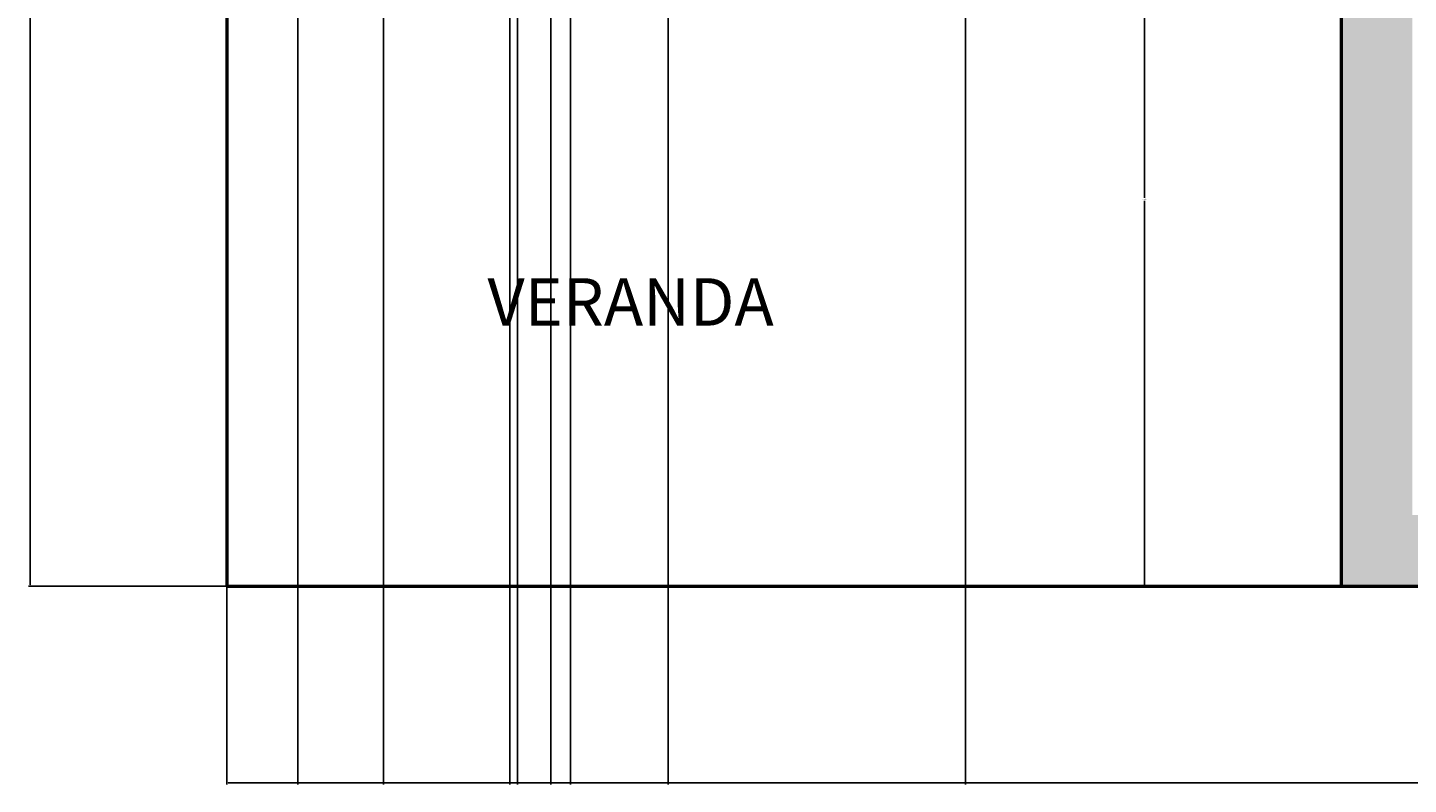
# Model space of a CAD drawing. Units: inches. Extents: x 3 to 380, y -485 to 60.
# Tile 1 of 8: x 3 to 177, y -485 to -390. Entities that reach past the tile are written whole.
import ezdxf

# ---------------------------------------------------------------- set-up
doc = ezdxf.new("R2010")
doc.units = ezdxf.units.IN
doc.header["$MEASUREMENT"] = 0
for name, color, linetype, lineweight in [('A-ANNO-DIMS', 2, 'Continuous', 18), ('A-AREA-IDEN', 7, 'Continuous', 25), ('A-WALL', 7, 'Continuous', 50), ('A-WALL-PATT', 252, 'Continuous', 13)]:
    doc.layers.add(name, color=color, linetype=linetype, lineweight=lineweight)
doc.styles.get("Standard").update_dxf_attribs({"font": 'arial.ttf'})
doc.dimstyles.get("Standard").update_dxf_attribs({"dimtxt": 0.18, "dimasz": 0.18, "dimexe": 0.18, "dimexo": 0.0625, "dimgap": 0.09, "dimtad": 0, "dimtih": 1, "dimtoh": 1, "dimdec": 0, "dimzin": 0, "dimdsep": 46, "dimlunit": 3, "dimtxsty": 'Standard', "dimcen": 0.09, "dimadec": 0, "dimazin": 0, "dimtfac": 1, "dimtdec": 0, "dimtofl": 0, "dimtmove": 0, "dimatfit": 3, "dimfxl": 1, "dimtolj": 1, "dimtzin": 0, "dimarcsym": 0})

# ---------------------------------------------------------------- blocks, each defined once
blk = doc.blocks.new('*D49')
at = {"layer": 'A-ANNO-DIMS', "color": 0, "lineweight": -2, "transparency": 16777216}
for p, q in [((27.84, -460.4), (27.84, -485.42)), ((354.84, -460.4), (354.84, -485.42)), ((28.02, -485.24), (191.05, -485.24)), ((354.66, -485.24), (191.63, -485.24))]:
    blk.add_line(p, q, dxfattribs=at)
at = {"layer": 'A-ANNO-DIMS', "color": 0, "transparency": 16777216}
for points in [[(28.02, -485.21), (28.02, -485.27), (27.84, -485.24)], [(354.66, -485.21), (354.66, -485.27), (354.84, -485.24)]]:
    blk.add_solid(points, dxfattribs=at)
at = {"layer": 'Defpoints', "color": 0, "transparency": 16777216}
for p in [(27.84, -460.34), (354.84, -460.34), (354.84, -485.24)]:
    blk.add_point(p, dxfattribs=at)
at = {"layer": 'A-ANNO-DIMS', "color": 0, "transparency": 16777216, "insert": (191.34, -485.24), "char_height": 0.18, "attachment_point": 5}
blk.add_mtext('\\A1;327', dxfattribs=at)
blk = doc.blocks.new('*D50')
at = {"layer": 'A-ANNO-DIMS', "color": 0, "lineweight": -2, "transparency": 16777216}
for p, q in [((27.78, 15.16), (2.76, 15.16)), ((2.94, 14.98), (2.94, -222.4)), ((2.94, -460.16), (2.94, -222.77)), ((27.78, -460.34), (2.76, -460.34))]:
    blk.add_line(p, q, dxfattribs=at)
at = {"layer": 'A-ANNO-DIMS', "color": 0, "transparency": 16777216}
for points in [[(2.91, 14.98), (2.97, 14.98), (2.94, 15.16)], [(2.91, -460.16), (2.97, -460.16), (2.94, -460.34)]]:
    blk.add_solid(points, dxfattribs=at)
at = {"layer": 'Defpoints', "color": 0, "transparency": 16777216}
for p in [(2.94, 15.16), (27.84, 15.16), (27.84, -460.34)]:
    blk.add_point(p, dxfattribs=at)
at = {"layer": 'A-ANNO-DIMS', "color": 0, "transparency": 16777216, "insert": (2.94, -222.59), "char_height": 0.18, "attachment_point": 5}
blk.add_mtext('\\A1;475.5', dxfattribs=at)
blk = doc.blocks.new('*D51')
at = {"layer": 'A-ANNO-DIMS', "color": 0, "lineweight": -2, "transparency": 16777216}
for p, q in [((151.9, 34.66), (379.92, 34.66)), ((379.74, 34.48), (379.74, -212.65)), ((379.74, -460.16), (379.74, -213.02)), ((354.9, -460.34), (379.92, -460.34))]:
    blk.add_line(p, q, dxfattribs=at)
at = {"layer": 'A-ANNO-DIMS', "color": 0, "transparency": 16777216}
for points in [[(379.71, 34.48), (379.77, 34.48), (379.74, 34.66)], [(379.71, -460.16), (379.77, -460.16), (379.74, -460.34)]]:
    blk.add_solid(points, dxfattribs=at)
at = {"layer": 'Defpoints', "color": 0, "transparency": 16777216}
for p in [(151.84, 34.66), (354.84, -460.34), (379.74, -460.34)]:
    blk.add_point(p, dxfattribs=at)
at = {"layer": 'A-ANNO-DIMS', "color": 0, "transparency": 16777216, "insert": (379.74, -212.84), "char_height": 0.18, "attachment_point": 5}
blk.add_mtext('\\A1;495', dxfattribs=at)
blk = doc.blocks.new('*D56')
at = {"layer": 'A-ANNO-DIMS', "color": 0, "lineweight": -2, "transparency": 16777216}
for p, q in [((168.78, -362.43), (143.76, -362.43)), ((143.94, -362.61), (143.94, -411.2)), ((143.94, -460.16), (143.94, -411.56)), ((168.78, -460.34), (143.76, -460.34))]:
    blk.add_line(p, q, dxfattribs=at)
at = {"layer": 'A-ANNO-DIMS', "color": 0, "transparency": 16777216}
for points in [[(143.91, -362.61), (143.97, -362.61), (143.94, -362.43)], [(143.91, -460.16), (143.97, -460.16), (143.94, -460.34)]]:
    blk.add_solid(points, dxfattribs=at)
at = {"layer": 'Defpoints', "color": 0, "transparency": 16777216}
for p in [(143.94, -362.43), (168.84, -362.43), (168.84, -460.34)]:
    blk.add_point(p, dxfattribs=at)
at = {"layer": 'A-ANNO-DIMS', "color": 0, "transparency": 16777216, "insert": (143.94, -411.38), "char_height": 0.18, "attachment_point": 5}
blk.add_mtext('\\A1;97.9', dxfattribs=at)
blk = doc.blocks.new('*D92')
at = {"layer": 'A-ANNO-DIMS', "color": 0, "lineweight": -2, "transparency": 16777216}
for p, q in [((36.84, -85.2), (36.84, -485.42)), ((63.65, -85.2), (63.65, -485.42)), ((37.02, -485.24), (49.87, -485.24)), ((63.47, -485.24), (50.62, -485.24))]:
    blk.add_line(p, q, dxfattribs=at)
at = {"layer": 'A-ANNO-DIMS', "color": 0, "transparency": 16777216}
for points in [[(37.02, -485.21), (37.02, -485.27), (36.84, -485.24)], [(63.47, -485.21), (63.47, -485.27), (63.65, -485.24)]]:
    blk.add_solid(points, dxfattribs=at)
at = {"layer": 'Defpoints', "color": 0, "transparency": 16777216}
for p in [(36.84, -85.14), (63.65, -85.14), (63.65, -485.24)]:
    blk.add_point(p, dxfattribs=at)
at = {"layer": 'A-ANNO-DIMS', "color": 0, "transparency": 16777216, "insert": (50.24, -485.24), "char_height": 0.18, "attachment_point": 5}
blk.add_mtext('\\A1;26.81', dxfattribs=at)
blk = doc.blocks.new('*D93')
at = {"layer": 'A-ANNO-DIMS', "color": 0, "lineweight": -2, "transparency": 16777216}
for p, q in [((71.32, -23.85), (71.32, -485.42)), ((121.32, -23.85), (121.32, -485.42)), ((71.5, -485.24), (95.92, -485.24)), ((121.14, -485.24), (96.72, -485.24))]:
    blk.add_line(p, q, dxfattribs=at)
at = {"layer": 'A-ANNO-DIMS', "color": 0, "transparency": 16777216}
for points in [[(71.5, -485.21), (71.5, -485.27), (71.32, -485.24)], [(121.14, -485.21), (121.14, -485.27), (121.32, -485.24)]]:
    blk.add_solid(points, dxfattribs=at)
at = {"layer": 'Defpoints', "color": 0, "transparency": 16777216}
for p in [(71.32, -23.79), (121.32, -23.79), (71.32, -485.24)]:
    blk.add_point(p, dxfattribs=at)
at = {"layer": 'A-ANNO-DIMS', "color": 0, "transparency": 16777216, "insert": (96.32, -485.24), "char_height": 0.18, "attachment_point": 5}
blk.add_mtext('\\A1;49.99', dxfattribs=at)
blk = doc.blocks.new('*D98')
at = {"layer": 'A-ANNO-DIMS', "color": 0, "lineweight": -2, "transparency": 16777216}
for p, q in [((47.67, -331.76), (47.67, -485.42)), ((64.61, -331.76), (64.61, -485.42)), ((47.85, -485.24), (55.68, -485.24)), ((64.43, -485.24), (56.59, -485.24))]:
    blk.add_line(p, q, dxfattribs=at)
at = {"layer": 'A-ANNO-DIMS', "color": 0, "transparency": 16777216}
for points in [[(47.85, -485.21), (47.85, -485.27), (47.67, -485.24)], [(64.43, -485.21), (64.43, -485.27), (64.61, -485.24)]]:
    blk.add_solid(points, dxfattribs=at)
at = {"layer": 'Defpoints', "color": 0, "transparency": 16777216}
for p in [(47.67, -331.7), (64.61, -331.7), (64.61, -485.24)]:
    blk.add_point(p, dxfattribs=at)
at = {"layer": 'A-ANNO-DIMS', "color": 0, "transparency": 16777216, "insert": (56.14, -485.24), "char_height": 0.18, "attachment_point": 5}
blk.add_mtext('\\A1;16.942', dxfattribs=at)
blk = doc.blocks.new('*D100')
at = {"layer": 'A-ANNO-DIMS', "color": 0, "lineweight": -2, "transparency": 16777216}
for p, q in [((68.84, -311.64), (68.84, -485.42)), ((83.67, -311.64), (83.67, -485.42)), ((69.02, -485.24), (75.8, -485.24)), ((83.49, -485.24), (76.71, -485.24))]:
    blk.add_line(p, q, dxfattribs=at)
at = {"layer": 'A-ANNO-DIMS', "color": 0, "transparency": 16777216}
for points in [[(69.02, -485.21), (69.02, -485.27), (68.84, -485.24)], [(83.49, -485.21), (83.49, -485.27), (83.67, -485.24)]]:
    blk.add_solid(points, dxfattribs=at)
at = {"layer": 'Defpoints', "color": 0, "transparency": 16777216}
for p in [(68.84, -311.58), (83.67, -311.58), (83.67, -485.24)]:
    blk.add_point(p, dxfattribs=at)
at = {"layer": 'A-ANNO-DIMS', "color": 0, "transparency": 16777216, "insert": (76.25, -485.24), "char_height": 0.18, "attachment_point": 5}
blk.add_mtext('\\A1;14.824', dxfattribs=at)

msp = doc.modelspace()

# ---------------------------------------------------------------- hatches: boundary and pattern name
at = {"layer": 'A-WALL-PATT'}
h = msp.add_hatch(color=256, dxfattribs=at)
h.dxf.hatch_style = 1
h.paths.add_polyline_path([(36.8404, 6.1643), (51.3404, 6.1643), (51.3404, 15.1643), (27.8404, 15.1643), (27.8404, -143.6318), (36.8404, -143.6318)])
h.paths.add_polyline_path([(125.8404, 10.6643), (125.8404, 15.1643), (111.3404, 15.1643), (111.3404, 6.1643), (125.8404, 6.1643)])
h.paths.add_polyline_path([(170.6358, 15.1643), (153.8404, 15.1643), (153.8404, 6.1643), (156.8404, 6.1643), (156.8404, -82.3357), (173.3404, -82.3357), (173.3404, -130.3357), (177.8404, -130.3357), (180.8404, -130.3357), (180.8404, -125.8357), (177.8404, -125.8357), (177.8404, -82.3357), (201.8404, -82.3357), (201.8404, -38.0857), (197.3404, -38.0857), (197.3404, -77.8357), (161.3404, -77.8357), (161.3404, 6.1643), (170.6358, 6.1643)])
h.paths.add_polyline_path([(241.3739, 15.1643), (194.6358, 15.1643), (194.6358, 6.1643), (241.3739, 6.1643)])
h.paths.add_polyline_path([(201.8404, 6.1643), (197.3404, 6.1643), (197.3404, -12.1977), (201.8404, -12.1977)], flags=17)
h.paths.add_polyline_path([(354.8404, 15.1643), (301.3739, 15.1643), (301.3739, 6.1643), (345.8404, 6.1643), (345.8404, -34.0336), (354.8404, -34.0336)])
h.paths.add_polyline_path([(354.8404, -94.0336), (345.8404, -94.0336), (345.8404, -159.3738), (354.8404, -159.3738)])
h.paths.add_polyline_path([(345.8404, -125.8357), (209.3404, -125.8357), (209.3404, -205.8357), (211.5904, -205.8357), (213.8404, -205.8357), (213.8404, -130.3357), (345.8404, -130.3357)])
h.paths.add_polyline_path([(36.8404, -203.6318), (27.8404, -203.6318), (27.8404, -270.1269), (36.8404, -270.1269)])
h.paths.add_polyline_path([(36.8404, -330.1269), (27.8404, -330.1269), (27.8404, -362.428), (57.3404, -362.428), (57.3404, -353.428), (36.8404, -353.428)])
h.paths.add_polyline_path([(177.8404, -331.3357), (180.8404, -331.3357), (180.8404, -326.8357), (173.3404, -326.8357), (173.3404, -353.428), (165.8404, -353.428), (165.8404, -362.428), (168.8404, -362.428), (168.8404, -451.3357), (168.8404, -460.3357), (231.8404, -460.3357), (231.8404, -451.3357), (177.8404, -451.3357)])
h.paths.add_polyline_path([(354.8404, -305.1003), (345.8404, -305.1003), (345.8404, -363.2829), (354.8404, -363.2829)])
h.paths.add_polyline_path([(345.8404, -326.8357), (213.8404, -326.8357), (213.8404, -312.8357), (211.5904, -312.8357), (209.3404, -312.8357), (209.3404, -331.3357), (345.8404, -331.3357)])
h.paths.add_polyline_path([(345.8404, -262.3357), (237.8404, -262.3357), (237.8404, -233.8357), (209.3404, -233.8357), (209.3404, -284.8357), (213.8404, -284.8357), (213.8404, -238.3357), (233.3404, -238.3357), (233.3404, -266.8357), (345.8404, -266.8357)])
h.paths.add_polyline_path([(354.8404, -219.3738), (345.8404, -219.3738), (345.8404, -281.1003), (354.8404, -281.1003)])

# ---------------------------------------------------------------- linework, layer by layer
at = {"layer": 'A-WALL'}
for p, q in [((27.8404, 15.1643), (27.8404, -460.3357)), ((168.8404, -362.428), (168.8404, -451.3357)), ((168.8404, -451.3357), (168.8404, -460.3357)), ((27.8404, -460.3357), (354.8404, -460.3357))]:
    msp.add_line(p, q, dxfattribs=at)

# ---------------------------------------------------------------- texts
at = {"layer": 'A-AREA-IDEN', "insert": (60.8169, -421.3749), "char_height": 6, "attachment_point": 1}
msp.add_mtext('VERANDA', dxfattribs=at)

# ---------------------------------------------------------------- dimensions: what is measured, and where the dimension line sits
at = {"layer": 'A-ANNO-DIMS'}
for base, p1, p2, override, picture, middle in [((379.7404, -460.3357), (151.8404, 34.6643), (354.8404, -460.3357), {"dimdec": 0, "dimlfac": 1, "dimrnd": 0, "dimzin": 0, "dimdsep": 46, "dimlunit": 2}, '*D51', (379.7404, -212.8357)), ((2.9404, 15.1643), (27.8404, -460.3357), (27.8404, 15.1643), {"dimdec": 1, "dimlfac": 1, "dimrnd": 0, "dimzin": 0, "dimdsep": 46, "dimlunit": 2}, '*D50', (2.9404, -222.5857)), ((143.9404, -362.428), (168.8404, -460.3357), (168.8404, -362.428), {"dimdec": 1, "dimlfac": 1, "dimrnd": 0, "dimzin": 0, "dimdsep": 46, "dimlunit": 2}, '*D56', (143.9404, -411.3818))]:
    dim = msp.add_linear_dim(base=base, p1=p1, p2=p2, angle=90, dimstyle='Standard', override=override, dxfattribs=at)
    dim.commit()
    dim.dimension.update_dxf_attribs({"geometry": picture, "text_midpoint": middle})
for base, p1, p2, override, picture, middle in [((71.3212, -485.2357), (121.3159, -23.7901), (71.3212, -23.7901), {"dimdec": 2, "dimlfac": 1, "dimrnd": 0, "dimzin": 0, "dimdsep": 46, "dimlunit": 2}, '*D93', (96.3185, -485.2357)), ((63.6489, -485.2357), (36.8404, -85.1388), (63.6489, -85.1388), {"dimdec": 2, "dimlfac": 1, "dimrnd": 0, "dimzin": 0, "dimdsep": 46, "dimlunit": 2}, '*D92', (50.2446, -485.2357)), ((83.6667, -485.2357), (68.8427, -311.5805), (83.6667, -311.5805), {"dimdec": 3, "dimlfac": 1, "dimrnd": 0, "dimzin": 0, "dimdsep": 46, "dimlunit": 2}, '*D100', (76.2547, -485.2357)), ((64.6072, -485.2357), (47.6655, -331.6989), (64.6072, -331.6989), {"dimdec": 3, "dimlfac": 1, "dimrnd": 0, "dimzin": 0, "dimdsep": 46, "dimlunit": 2}, '*D98', (56.1364, -485.2357)), ((354.8404, -485.2357), (27.8404, -460.3357), (354.8404, -460.3357), {"dimdec": 0, "dimlfac": 1, "dimrnd": 0, "dimzin": 0, "dimdsep": 46, "dimlunit": 2}, '*D49', (191.3404, -485.2357))]:
    dim = msp.add_linear_dim(base=base, p1=p1, p2=p2, dimstyle='Standard', override=override, dxfattribs=at)
    dim.commit()
    dim.dimension.update_dxf_attribs({"geometry": picture, "text_midpoint": middle})

doc.saveas('drawing.dxf')
